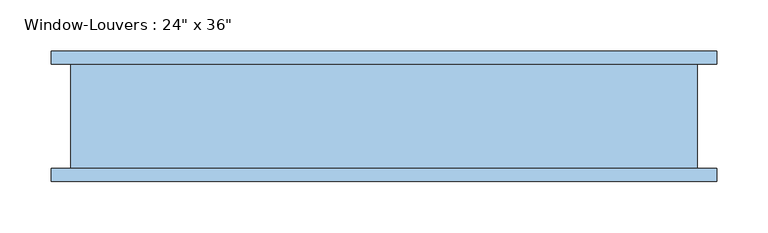
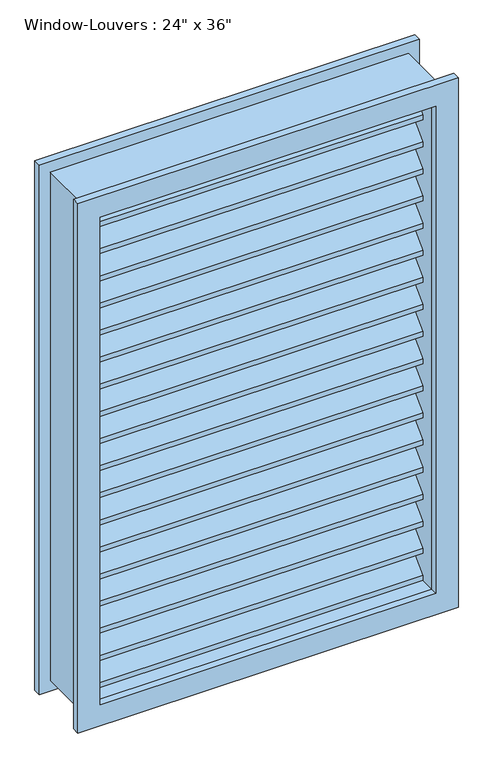
"""IFC4 building model written with IfcOpenShell, lengths in millimetres: window geometry."""

from ifc_helpers import new_model, si_unit, frame, origin, place, context, project, spatial, polyline, outline, extrude, source, transform, mapped, element, save


def window_d9a389d2(model_context):
    return source(origin(), model_context, "Body", "SweptSolid", [
        extrude(outline(polyline([(44.45, 1722.872368), (44.45, 1713.8921119), (6.35, 1751.9921119), (-31.75, 1713.8921119), (-31.75, 1722.872368), (6.35, 1760.972368), (44.45, 1722.872368)])), frame((-285.75, 0.0, 0.0), z_axis=(1.0, 0.0, 0.0), x_axis=(0.0, 1.0, 0.0)), (0.0, 0.0, 1.0), 571.5),
        extrude(outline(polyline([(44.45, 1674.094736), (44.45, 1665.1144799), (6.35, 1703.2144799), (-31.75, 1665.1144799), (-31.75, 1674.094736), (6.35, 1712.194736), (44.45, 1674.094736)])), frame((-285.75, 0.0, 0.0), z_axis=(1.0, 0.0, 0.0), x_axis=(0.0, 1.0, 0.0)), (0.0, 0.0, 1.0), 571.5),
        extrude(outline(polyline([(44.45, 1625.317104), (44.45, 1616.3368479), (6.35, 1654.4368479), (-31.75, 1616.3368479), (-31.75, 1625.317104), (6.35, 1663.417104), (44.45, 1625.317104)])), frame((-285.75, 0.0, 0.0), z_axis=(1.0, 0.0, 0.0), x_axis=(0.0, 1.0, 0.0)), (0.0, 0.0, 1.0), 571.5),
        extrude(outline(polyline([(44.45, 1576.539472), (44.45, 1567.5592159), (6.35, 1605.6592159), (-31.75, 1567.5592159), (-31.75, 1576.539472), (6.35, 1614.639472), (44.45, 1576.539472)])), frame((-285.75, 0.0, 0.0), z_axis=(1.0, 0.0, 0.0), x_axis=(0.0, 1.0, 0.0)), (0.0, 0.0, 1.0), 571.5),
        extrude(outline(polyline([(44.45, 1527.76184), (44.45, 1518.7815839), (6.35, 1556.8815839), (-31.75, 1518.7815839), (-31.75, 1527.76184), (6.35, 1565.86184), (44.45, 1527.76184)])), frame((-285.75, 0.0, 0.0), z_axis=(1.0, 0.0, 0.0), x_axis=(0.0, 1.0, 0.0)), (0.0, 0.0, 1.0), 571.5),
        extrude(outline(polyline([(44.45, 1478.984208), (44.45, 1470.0039519), (6.35, 1508.1039519), (-31.75, 1470.0039519), (-31.75, 1478.984208), (6.35, 1517.084208), (44.45, 1478.984208)])), frame((-285.75, 0.0, 0.0), z_axis=(1.0, 0.0, 0.0), x_axis=(0.0, 1.0, 0.0)), (0.0, 0.0, 1.0), 571.5),
        extrude(outline(polyline([(44.45, 1430.206576), (44.45, 1421.2263199), (6.35, 1459.3263199), (-31.75, 1421.2263199), (-31.75, 1430.206576), (6.35, 1468.306576), (44.45, 1430.206576)])), frame((-285.75, 0.0, 0.0), z_axis=(1.0, 0.0, 0.0), x_axis=(0.0, 1.0, 0.0)), (0.0, 0.0, 1.0), 571.5),
        extrude(outline(polyline([(44.45, 1381.4289441), (44.45, 1372.4486879), (6.35, 1410.5486879), (-31.75, 1372.4486879), (-31.75, 1381.4289441), (6.35, 1419.5289441), (44.45, 1381.4289441)])), frame((-285.75, 0.0, 0.0), z_axis=(1.0, 0.0, 0.0), x_axis=(0.0, 1.0, 0.0)), (0.0, 0.0, 1.0), 571.5),
        extrude(outline(polyline([(44.45, 1332.6513121), (44.45, 1323.6710559), (6.35, 1361.7710559), (-31.75, 1323.6710559), (-31.75, 1332.6513121), (6.35, 1370.7513121), (44.45, 1332.6513121)])), frame((-285.75, 0.0, 0.0), z_axis=(1.0, 0.0, 0.0), x_axis=(0.0, 1.0, 0.0)), (0.0, 0.0, 1.0), 571.5),
        extrude(outline(polyline([(44.45, 1283.8736801), (44.45, 1274.893424), (6.35, 1312.993424), (-31.75, 1274.893424), (-31.75, 1283.8736801), (6.35, 1321.9736801), (44.45, 1283.8736801)])), frame((-285.75, 0.0, 0.0), z_axis=(1.0, 0.0, 0.0), x_axis=(0.0, 1.0, 0.0)), (0.0, 0.0, 1.0), 571.5),
        extrude(outline(polyline([(44.45, 1235.0960481), (44.45, 1226.115792), (6.35, 1264.215792), (-31.75, 1226.115792), (-31.75, 1235.0960481), (6.35, 1273.1960481), (44.45, 1235.0960481)])), frame((-285.75, 0.0, 0.0), z_axis=(1.0, 0.0, 0.0), x_axis=(0.0, 1.0, 0.0)), (0.0, 0.0, 1.0), 571.5),
        extrude(outline(polyline([(44.45, 1186.3184161), (44.45, 1177.33816), (6.35, 1215.43816), (-31.75, 1177.33816), (-31.75, 1186.3184161), (6.35, 1224.4184161), (44.45, 1186.3184161)])), frame((-285.75, 0.0, 0.0), z_axis=(1.0, 0.0, 0.0), x_axis=(0.0, 1.0, 0.0)), (0.0, 0.0, 1.0), 571.5),
        extrude(outline(polyline([(44.45, 1137.5407841), (44.45, 1128.560528), (6.35, 1166.660528), (-31.75, 1128.560528), (-31.75, 1137.5407841), (6.35, 1175.6407841), (44.45, 1137.5407841)])), frame((-285.75, 0.0, 0.0), z_axis=(1.0, 0.0, 0.0), x_axis=(0.0, 1.0, 0.0)), (0.0, 0.0, 1.0), 571.5),
        extrude(outline(polyline([(44.45, 1088.7631521), (44.45, 1079.782896), (6.35, 1117.882896), (-31.75, 1079.782896), (-31.75, 1088.7631521), (6.35, 1126.8631521), (44.45, 1088.7631521)])), frame((-285.75, 0.0, 0.0), z_axis=(1.0, 0.0, 0.0), x_axis=(0.0, 1.0, 0.0)), (0.0, 0.0, 1.0), 571.5),
        extrude(outline(polyline([(44.45, 1039.9855201), (44.45, 1031.005264), (6.35, 1069.105264), (-31.75, 1031.005264), (-31.75, 1039.9855201), (6.35, 1078.0855201), (44.45, 1039.9855201)])), frame((-285.75, 0.0, 0.0), z_axis=(1.0, 0.0, 0.0), x_axis=(0.0, 1.0, 0.0)), (0.0, 0.0, 1.0), 571.5),
        extrude(outline(polyline([(44.45, 991.2078881), (44.45, 982.227632), (6.35, 1020.327632), (-31.75, 982.227632), (-31.75, 991.2078881), (6.35, 1029.3078881), (44.45, 991.2078881)])), frame((-285.75, 0.0, 0.0), z_axis=(1.0, 0.0, 0.0), x_axis=(0.0, 1.0, 0.0)), (0.0, 0.0, 1.0), 571.5),
        extrude(outline(polyline([(44.45, 1771.65), (44.45, 1762.6697439), (6.35, 1800.7697439), (-31.75, 1762.6697439), (-31.75, 1771.65), (6.35, 1809.75), (44.45, 1771.65)])), frame((-285.75, 0.0, 0.0), z_axis=(1.0, 0.0, 0.0), x_axis=(0.0, 1.0, 0.0)), (0.0, 0.0, 1.0), 571.5),
        extrude(outline(polyline([(44.45, 942.4302561), (44.45, 933.45), (6.35, 971.55), (-31.75, 933.45), (-31.75, 942.4302561), (6.35, 980.5302561), (44.45, 942.4302561)])), frame((-285.75, 0.0, 0.0), z_axis=(1.0, 0.0, 0.0), x_axis=(0.0, 1.0, 0.0)), (0.0, 0.0, 1.0), 571.5),
        extrude(outline(polyline([(1828.8, 304.8), (1828.8, -304.8), (914.4, -304.8), (914.4, 304.8), (1828.8, 304.8)]), holes=[polyline([(1809.75, 285.75), (933.45, 285.75), (933.45, -285.75), (1809.75, -285.75), (1809.75, 285.75)])]), frame((0.0, -57.15, 0.0), z_axis=(0.0, 1.0, 0.0), x_axis=(0.0, 0.0, 1.0)), (0.0, 0.0, 1.0), 101.6),
        extrude(outline(polyline([(1847.85, 323.85), (1847.85, -323.85), (895.35, -323.85), (895.35, 323.85), (1847.85, 323.85)]), holes=[polyline([(1809.75, 285.75), (933.45, 285.75), (933.45, -285.75), (1809.75, -285.75), (1809.75, 285.75)])]), frame((0.0, -69.85, 0.0), z_axis=(0.0, 1.0, 0.0), x_axis=(0.0, 0.0, 1.0)), (0.0, 0.0, 1.0), 12.7),
        extrude(outline(polyline([(1847.85, -323.85), (895.35, -323.85), (895.35, 323.85), (1847.85, 323.85), (1847.85, -323.85)]), holes=[polyline([(1809.75, -285.75), (1809.75, 285.75), (933.45, 285.75), (933.45, -285.75), (1809.75, -285.75)])]), frame((0.0, 44.45, 0.0), z_axis=(0.0, 1.0, 0.0), x_axis=(0.0, 0.0, 1.0)), (0.0, 0.0, 1.0), 12.7),
    ])


if __name__ == "__main__":
    model = new_model("IFC4")
    model_context = context("Model", 3, world=origin())
    ifc_project = project(units=[si_unit("LENGTHUNIT", "METRE", prefix="MILLI")], contexts=[model_context])
    site = spatial("IfcSite", under=ifc_project)
    building = spatial("IfcBuilding", under=site)
    placement = place(None, origin())
    window_shape = window_d9a389d2(model_context)
    element("IfcWindow", 1, ObjectType="Window-Louvers : 24\" x 36\"", at=placement, inside=building, context=model_context, shape_type="MappedRepresentation", body=[
        mapped(window_shape, transform((0.0, 0.0, 0.0), x_axis=(1.0, 0.0, 0.0), y_axis=(0.0, 1.0, 0.0), z_axis=(0.0, 0.0, 1.0))),
    ])
    save(model, "model.ifc")

# Revit data of these elements
# Type "Window-Louvers : 24\" x 36\""
#   Type Mark = "20"
#   Construction Type Id = "GSP4R"
#   Assembly Code = "B20"
#   Analytic Construction = "1/8 in Pilkington single glazing"
#   Visual Light Transmittance = 0.9
#   Thermal Resistance (R) = 1.53941 (h·ft²·°F)/BTU
#   Solar Heat Gain Coefficient = 0.78
#   Max Height = 3' - 0.71751"
#   Height = 3' - 0"
#   Heat Transfer Coefficient (U) = 0.6496 BTU/(h·ft²·°F)
#   Blade Width [instance default] = 1' - 10 1/2"
#   Blade Vertical Thickness = 0' - 0.35355"
#   Blade Thickness = 0' - 0 1/4"
#   Blade Spacing = 0' - 1 1/2"
#   Blade Height = 0' - 1.85355"
#   Blade Depth = 0' - 3"
#   Blade Angle = 45.00°
#   Default Sill Height = 3' - 0"
#   Trim Projection_Exterior = 0' - 0 1/2"
#   Trim Projection_Interior = 0' - 0 1/2"
#   Trim Width_Exterior = 0' - 1 1/2"
#   Trim Width_Interior = 0' - 1 1/2"
#   Width = 2' - 0"
#   Max Blade Count = 19
#   Define Thermal Properties by = 1
#   Blade Count = 18
#   Frame Material = Birch
#   Louver Material = Birch
#   Trim Exterior Material = Birch
#   Trim Interior Material = Birch
#   Wall Closure = (empty or 0)
# Element 1 (IfcWindow, "Window-Louvers : 24\" x 36\"")
#   Materials on its faces: "Birch"
# Materials
#   "Birch": class "Wood", colour RGB 224 178 126, transparency 0, Description = "Betula Alleghaniensis", Cost = 0
